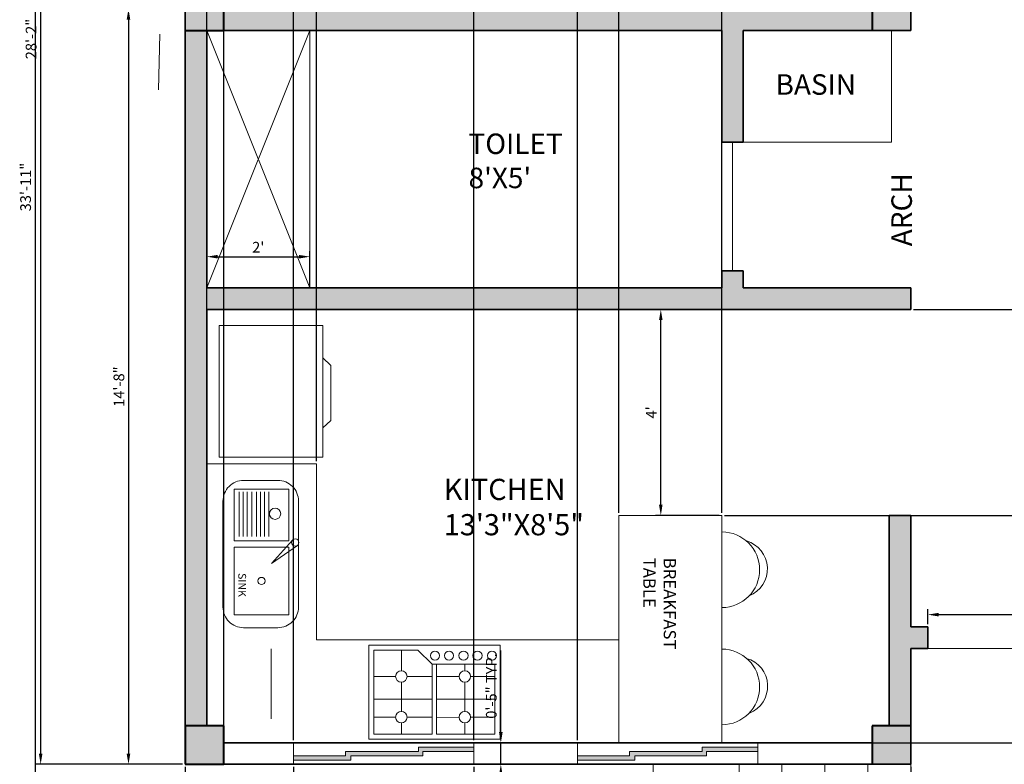
# Model space of a CAD drawing. Units: inches. Extents: x 918 to 1328, y 603 to 1174.
# Tile 2 of 4: x 918 to 1147, y 798 to 972. Entities that reach past the tile are written whole.
import ezdxf

# ---------------------------------------------------------------- set-up
doc = ezdxf.new("R2010")
doc.units = ezdxf.units.IN
for name, color, linetype, lineweight in [('A-ANNO-DIMS', 1, 'Continuous', 18), ('A-ANNO-TEXT', 7, 'Continuous', 18), ('A-COLS', 7, 'Continuous', 40), ('A-DETL', 8, 'Continuous', 13), ('A-DOOR', 4, 'Continuous', 18), ('A-FLOR-CASE', 8, 'Continuous', 20), ('A-FURN', 8, 'Continuous', 18), ('A-GLAZ', 4, 'Continuous', 18), ('A-GLAZ-PATT', 5, 'Continuous', 13), ('A-WALL', 7, 'Continuous', 35), ('A-WALL-PATT', 7, 'Continuous', 13)]:
    doc.layers.add(name, color=color, linetype=linetype, lineweight=lineweight)
for name, color, linetype, lineweight, true_color in [('A-AREA-IDEN', 251, 'Continuous', 20, 0x636466), ('A-COLS-PATT', 251, 'Continuous', 13, 0x636466), ('A-EQPM', 252, 'Continuous', 18, 0x939598), ('A-FLOR-FIXT', 252, 'Continuous', 18, 0x939598), ('A-FLOR-STRS', 251, 'Continuous', 20, 0x636466)]:
    doc.layers.add(name, color=color, linetype=linetype, lineweight=lineweight, true_color=true_color)
doc.styles.get("Standard").update_dxf_attribs({"font": 'arial.ttf'})
doc.dimstyles.new('ISO-25', dxfattribs={"dimtxt": 2.5, "dimasz": 2.5, "dimexe": 1.25, "dimexo": 0.625, "dimtad": 1, "dimdec": 0, "dimlunit": 3, "dimtxsty": 'Standard', "dimcen": 2.5, "dimadec": 0, "dimazin": 0, "dimtfac": 1, "dimtdec": 0, "dimtmove": 0, "dimatfit": 3, "dimfxl": 1, "dimarcsym": 0})

# ---------------------------------------------------------------- blocks, each defined once
blk = doc.blocks.new('*D2')
at = {"layer": 'A-ANNO-DIMS', "color": 0, "lineweight": -2, "transparency": 16777216}
for p, q in [((955.86, 1136.24), (921.53, 1136.24)), ((922.78, 1133.74), (922.78, 800.74)), ((955.86, 798.24), (921.53, 798.24))]:
    blk.add_line(p, q, dxfattribs=at)
at = {"layer": 'A-ANNO-DIMS', "color": 0, "transparency": 16777216}
for points in [[(922.37, 1133.74), (923.2, 1133.74), (922.78, 1136.24)], [(922.37, 800.74), (923.2, 800.74), (922.78, 798.24)]]:
    blk.add_solid(points, dxfattribs=at)
at = {"layer": 'Defpoints', "color": 0, "transparency": 16777216}
for p in [(956.48, 1136.24), (922.78, 798.24), (956.48, 798.24)]:
    blk.add_point(p, dxfattribs=at)
at = {"layer": 'A-ANNO-DIMS', "color": 0, "transparency": 16777216, "insert": (920.88, 967.24), "char_height": 2.5, "attachment_point": 5, "rotation": 90}
blk.add_mtext('28\'-2"', dxfattribs=at)
blk = doc.blocks.new('*D3')
at = {"layer": 'A-ANNO-DIMS', "color": 0, "lineweight": -2, "transparency": 16777216}
for p, q in [((961.48, 909.87), (961.48, 917.77)), ((985.48, 909.87), (985.48, 917.77)), ((963.98, 916.52), (982.98, 916.52))]:
    blk.add_line(p, q, dxfattribs=at)
at = {"layer": 'A-ANNO-DIMS', "color": 0, "transparency": 16777216}
for points in [[(963.98, 916.93), (963.98, 916.1), (961.48, 916.52)], [(982.98, 916.93), (982.98, 916.1), (985.48, 916.52)]]:
    blk.add_solid(points, dxfattribs=at)
at = {"layer": 'Defpoints', "color": 0, "transparency": 16777216}
for p in [(985.48, 916.52), (961.48, 909.24), (985.48, 909.24)]:
    blk.add_point(p, dxfattribs=at)
at = {"layer": 'A-ANNO-DIMS', "color": 0, "transparency": 16777216, "insert": (973.48, 918.4), "char_height": 2.5, "attachment_point": 5}
blk.add_mtext("2'", dxfattribs=at)
blk = doc.blocks.new('*D8')
at = {"layer": 'A-ANNO-DIMS', "color": 0, "lineweight": -2, "transparency": 16777216}
for p, q in [((955.86, 974.24), (941.99, 974.24)), ((943.24, 971.74), (943.24, 800.74)), ((955.86, 798.24), (941.99, 798.24))]:
    blk.add_line(p, q, dxfattribs=at)
at = {"layer": 'A-ANNO-DIMS', "color": 0, "transparency": 16777216}
for points in [[(942.82, 971.74), (943.66, 971.74), (943.24, 974.24)], [(942.82, 800.74), (943.66, 800.74), (943.24, 798.24)]]:
    blk.add_solid(points, dxfattribs=at)
at = {"layer": 'Defpoints', "color": 0, "transparency": 16777216}
for p in [(956.48, 974.24), (943.24, 798.24), (956.48, 798.24)]:
    blk.add_point(p, dxfattribs=at)
at = {"layer": 'A-ANNO-DIMS', "color": 0, "transparency": 16777216, "insert": (941.34, 886.24), "char_height": 2.5, "attachment_point": 5, "rotation": 90}
blk.add_mtext('14\'-8"', dxfattribs=at)
blk = doc.blocks.new('*D11')
at = {"layer": 'A-ANNO-DIMS', "color": 0, "lineweight": -2, "transparency": 16777216}
for p, q in [((956.48, 797.62), (956.48, 707.87)), ((1125.48, 797.62), (1125.48, 707.87)), ((958.98, 709.12), (1122.98, 709.12))]:
    blk.add_line(p, q, dxfattribs=at)
at = {"layer": 'A-ANNO-DIMS', "color": 0, "transparency": 16777216}
for points in [[(958.98, 709.53), (958.98, 708.7), (956.48, 709.12)], [(1122.98, 709.53), (1122.98, 708.7), (1125.48, 709.12)]]:
    blk.add_solid(points, dxfattribs=at)
at = {"layer": 'Defpoints', "color": 0, "transparency": 16777216}
for p in [(956.48, 798.24), (1125.48, 798.24), (1125.48, 709.12)]:
    blk.add_point(p, dxfattribs=at)
at = {"layer": 'A-ANNO-DIMS', "color": 0, "transparency": 16777216, "insert": (1040.98, 711), "char_height": 2.5, "attachment_point": 5}
blk.add_mtext('14\'-1"', dxfattribs=at)
blk = doc.blocks.new('*D17')
at = {"layer": 'A-ANNO-DIMS', "color": 0, "lineweight": -2, "transparency": 16777216}
for p, q in [((1129.48, 830.87), (1129.48, 834.37)), ((1131.98, 833.12), (1174.98, 833.12)), ((1177.48, 830.87), (1177.48, 834.37))]:
    blk.add_line(p, q, dxfattribs=at)
at = {"layer": 'A-ANNO-DIMS', "color": 0, "transparency": 16777216}
for points in [[(1131.98, 833.53), (1131.98, 832.7), (1129.48, 833.12)], [(1174.98, 833.53), (1174.98, 832.7), (1177.48, 833.12)]]:
    blk.add_solid(points, dxfattribs=at)
at = {"layer": 'Defpoints', "color": 0, "transparency": 16777216}
for p in [(1177.48, 833.12), (1129.48, 830.24), (1177.48, 830.24)]:
    blk.add_point(p, dxfattribs=at)
at = {"layer": 'A-ANNO-DIMS', "color": 0, "transparency": 16777216, "insert": (1153.48, 834.99), "char_height": 2.5, "attachment_point": 5}
blk.add_mtext("4'", dxfattribs=at)
blk = doc.blocks.new('*D18')
at = {"layer": 'A-ANNO-DIMS', "color": 0, "lineweight": -2, "transparency": 16777216}
for p, q in [((1080.86, 904.24), (1066.01, 904.24)), ((1067.26, 858.74), (1067.26, 901.74)), ((1080.86, 856.24), (1066.01, 856.24))]:
    blk.add_line(p, q, dxfattribs=at)
at = {"layer": 'A-ANNO-DIMS', "color": 0, "transparency": 16777216}
for points in [[(1066.84, 901.74), (1067.67, 901.74), (1067.26, 904.24)], [(1066.84, 858.74), (1067.67, 858.74), (1067.26, 856.24)]]:
    blk.add_solid(points, dxfattribs=at)
at = {"layer": 'Defpoints', "color": 0, "transparency": 16777216}
for p in [(1067.26, 904.24), (1081.48, 904.24), (1081.48, 856.24)]:
    blk.add_point(p, dxfattribs=at)
at = {"layer": 'A-ANNO-DIMS', "color": 0, "transparency": 16777216, "insert": (1065.38, 880.24), "char_height": 2.5, "attachment_point": 5, "rotation": 90}
blk.add_mtext("4'", dxfattribs=at)
blk = doc.blocks.new('WIN-SLIDING-42')
for p, q in [((0, 5), (0, 0)), ((42, 5), (0, 5)), ((42, 0), (42, 5)), ((12.14, 3), (29.09, 3)), ((12.14, 1.97), (12.14, 3)), ((29.09, 3), (29.09, 4.02)), ((29.09, 4.02), (42, 4.02)), ((30.11, 1.97), (30.11, 3)), ((30.11, 3), (42, 3)), ((0, 1.97), (12.14, 1.97)), ((0, 0.97), (13.35, 0.97)), ((0, 0), (42, 0)), ((13.35, 0.97), (13.35, 1.97)), ((13.35, 1.97), (30.11, 1.97))]:
    blk.add_line(p, q)
blk = doc.blocks.new('*D32')
at = {"layer": 'A-ANNO-DIMS', "color": 0, "lineweight": -2, "transparency": 16777216}
for p, q in [((981.69, 797.62), (981.69, 790.69)), ((1023.69, 797.62), (1023.69, 790.69)), ((984.19, 791.94), (1021.19, 791.94)), ((1023.69, 791.94), (1073.9, 791.94))]:
    blk.add_line(p, q, dxfattribs=at)
at = {"layer": 'A-ANNO-DIMS', "color": 0, "transparency": 16777216}
for points in [[(984.19, 792.36), (984.19, 791.53), (981.69, 791.94)], [(1021.19, 792.36), (1021.19, 791.53), (1023.69, 791.94)]]:
    blk.add_solid(points, dxfattribs=at)
at = {"layer": 'Defpoints', "color": 0, "transparency": 16777216}
for p in [(981.69, 798.24), (1023.69, 798.24), (1023.69, 791.94)]:
    blk.add_point(p, dxfattribs=at)
at = {"layer": 'A-ANNO-DIMS', "color": 0, "transparency": 16777216, "insert": (1050.05, 793.86), "char_height": 2.5, "attachment_point": 5}
blk.add_mtext('SLIDING WINDOW 3\'-6" TYP.', dxfattribs=at)
blk = doc.blocks.new('*D33')
at = {"layer": 'A-ANNO-DIMS', "color": 0, "lineweight": -2, "transparency": 16777216}
for p, q in [((1029.99, 805.74), (1029.99, 824.73)), ((1024.31, 803.24), (1031.24, 803.24)), ((1029.99, 798.24), (1029.99, 803.24)), ((1024.31, 798.24), (1031.24, 798.24)), ((1029.99, 795.74), (1029.99, 793.24))]:
    blk.add_line(p, q, dxfattribs=at)
at = {"layer": 'A-ANNO-DIMS', "color": 0, "transparency": 16777216}
for points in [[(1029.57, 805.74), (1030.41, 805.74), (1029.99, 803.24)], [(1029.57, 795.74), (1030.41, 795.74), (1029.99, 798.24)]]:
    blk.add_solid(points, dxfattribs=at)
at = {"layer": 'Defpoints', "color": 0, "transparency": 16777216}
for p in [(1023.69, 803.24), (1029.99, 803.24), (1023.69, 798.24)]:
    blk.add_point(p, dxfattribs=at)
at = {"layer": 'A-ANNO-DIMS', "color": 0, "transparency": 16777216, "insert": (1028.09, 816.49), "char_height": 2.5, "attachment_point": 5, "rotation": 90}
blk.add_mtext('0\'-5" TYP.', dxfattribs=at)
blk = doc.blocks.new('*D44')
at = {"layer": 'A-ANNO-DIMS', "color": 0, "lineweight": -2, "transparency": 16777216}
for p, q in [((955.86, 1136.24), (920.25, 1136.24)), ((921.5, 1133.74), (921.5, 731.74)), ((1064.86, 729.24), (920.25, 729.24))]:
    blk.add_line(p, q, dxfattribs=at)
at = {"layer": 'A-ANNO-DIMS', "color": 0, "transparency": 16777216}
for points in [[(921.09, 1133.74), (921.92, 1133.74), (921.5, 1136.24)], [(921.09, 731.74), (921.92, 731.74), (921.5, 729.24)]]:
    blk.add_solid(points, dxfattribs=at)
at = {"layer": 'Defpoints', "color": 0, "transparency": 16777216}
for p in [(956.48, 1136.24), (921.5, 729.24), (1065.48, 729.24)]:
    blk.add_point(p, dxfattribs=at)
at = {"layer": 'A-ANNO-DIMS', "color": 0, "transparency": 16777216, "insert": (919.6, 932.74), "char_height": 2.5, "attachment_point": 5, "rotation": 90}
blk.add_mtext('33\'-11"', dxfattribs=at)
blk = doc.blocks.new('*D47')
at = {"layer": 'A-ANNO-DIMS', "color": 0, "lineweight": -2, "transparency": 16777216}
for p, q in [((965.48, 803.87), (965.48, 1166.19)), ((981.69, 803.87), (981.69, 1166.19)), ((967.98, 1164.94), (979.19, 1164.94))]:
    blk.add_line(p, q, dxfattribs=at)
at = {"layer": 'A-ANNO-DIMS', "color": 0, "transparency": 16777216}
for points in [[(967.98, 1165.36), (967.98, 1164.53), (965.48, 1164.94)], [(979.19, 1165.36), (979.19, 1164.53), (981.69, 1164.94)]]:
    blk.add_solid(points, dxfattribs=at)
at = {"layer": 'Defpoints', "color": 0, "transparency": 16777216}
for p in [(981.69, 1164.94), (965.48, 803.24), (981.69, 803.24)]:
    blk.add_point(p, dxfattribs=at)
at = {"layer": 'A-ANNO-DIMS', "color": 0, "transparency": 16777216, "insert": (973.59, 1166.82), "char_height": 2.5, "attachment_point": 5}
blk.add_mtext('1\'-4"', dxfattribs=at)
blk = doc.blocks.new('*D48')
at = {"layer": 'A-ANNO-DIMS', "color": 0, "lineweight": -2, "transparency": 16777216}
for p, q in [((1023.69, 803.87), (1023.69, 1166.19)), ((1047.83, 803.87), (1047.83, 1166.19)), ((1026.19, 1164.94), (1045.33, 1164.94))]:
    blk.add_line(p, q, dxfattribs=at)
at = {"layer": 'A-ANNO-DIMS', "color": 0, "transparency": 16777216}
for points in [[(1026.19, 1165.36), (1026.19, 1164.53), (1023.69, 1164.94)], [(1045.33, 1165.36), (1045.33, 1164.53), (1047.83, 1164.94)]]:
    blk.add_solid(points, dxfattribs=at)
at = {"layer": 'Defpoints', "color": 0, "transparency": 16777216}
for p in [(1047.83, 1164.94), (1023.69, 803.24), (1047.83, 803.24)]:
    blk.add_point(p, dxfattribs=at)
at = {"layer": 'A-ANNO-DIMS', "color": 0, "transparency": 16777216, "insert": (1035.76, 1166.84), "char_height": 2.5, "attachment_point": 5}
blk.add_mtext('2\'-0"', dxfattribs=at)
blk = doc.blocks.new('*D51')
at = {"layer": 'A-ANNO-DIMS', "color": 0, "lineweight": -2, "transparency": 16777216}
for p, q in [((1126.11, 904.24), (1321.43, 904.24)), ((1320.18, 901.74), (1320.18, 858.74)), ((1126.11, 856.24), (1321.43, 856.24))]:
    blk.add_line(p, q, dxfattribs=at)
at = {"layer": 'A-ANNO-DIMS', "color": 0, "transparency": 16777216}
for points in [[(1319.77, 901.74), (1320.6, 901.74), (1320.18, 904.24)], [(1319.77, 858.74), (1320.6, 858.74), (1320.18, 856.24)]]:
    blk.add_solid(points, dxfattribs=at)
at = {"layer": 'Defpoints', "color": 0, "transparency": 16777216}
for p in [(1125.48, 904.24), (1125.48, 856.24), (1320.18, 856.24)]:
    blk.add_point(p, dxfattribs=at)
at = {"layer": 'A-ANNO-DIMS', "color": 0, "transparency": 16777216, "insert": (1318.28, 880.24), "char_height": 2.5, "attachment_point": 5, "rotation": 90}
blk.add_mtext('4\'-0"', dxfattribs=at)
blk = doc.blocks.new('*D54')
at = {"layer": 'A-ANNO-DIMS', "color": 0, "lineweight": -2, "transparency": 16777216}
for p, q in [((961.48, 868.87), (961.48, 1166.19)), ((987.08, 868.87), (987.08, 1166.19)), ((963.98, 1164.94), (984.58, 1164.94))]:
    blk.add_line(p, q, dxfattribs=at)
at = {"layer": 'A-ANNO-DIMS', "color": 0, "transparency": 16777216}
for points in [[(963.98, 1165.36), (963.98, 1164.53), (961.48, 1164.94)], [(984.58, 1165.36), (984.58, 1164.53), (987.08, 1164.94)]]:
    blk.add_solid(points, dxfattribs=at)
at = {"layer": 'Defpoints', "color": 0, "transparency": 16777216}
for p in [(987.08, 1164.94), (961.48, 868.24), (987.08, 868.24)]:
    blk.add_point(p, dxfattribs=at)
at = {"layer": 'A-ANNO-DIMS', "color": 0, "transparency": 16777216, "insert": (974.28, 1166.86), "char_height": 2.5, "attachment_point": 5}
blk.add_mtext('2\'-1 1/2"', dxfattribs=at)
blk = doc.blocks.new('*D55')
at = {"layer": 'A-ANNO-DIMS', "color": 0, "lineweight": -2, "transparency": 16777216}
for p, q in [((1057.48, 856.87), (1057.48, 1166.19)), ((1081.48, 856.87), (1081.48, 1166.19)), ((1059.98, 1164.94), (1078.98, 1164.94))]:
    blk.add_line(p, q, dxfattribs=at)
at = {"layer": 'A-ANNO-DIMS', "color": 0, "transparency": 16777216}
for points in [[(1059.98, 1165.36), (1059.98, 1164.53), (1057.48, 1164.94)], [(1078.98, 1165.36), (1078.98, 1164.53), (1081.48, 1164.94)]]:
    blk.add_solid(points, dxfattribs=at)
at = {"layer": 'Defpoints', "color": 0, "transparency": 16777216}
for p in [(1081.48, 1164.94), (1057.48, 856.24), (1081.48, 856.24)]:
    blk.add_point(p, dxfattribs=at)
at = {"layer": 'A-ANNO-DIMS', "color": 0, "transparency": 16777216, "insert": (1069.48, 1166.84), "char_height": 2.5, "attachment_point": 5}
blk.add_mtext('2\'-0"', dxfattribs=at)
blk = doc.blocks.new('*D56')
at = {"layer": 'A-ANNO-DIMS', "color": 0, "lineweight": -2, "transparency": 16777216}
for p, q in [((1082.11, 856.24), (1321.43, 856.24)), ((1320.18, 853.74), (1320.18, 805.74)), ((1082.11, 803.24), (1321.43, 803.24))]:
    blk.add_line(p, q, dxfattribs=at)
at = {"layer": 'A-ANNO-DIMS', "color": 0, "transparency": 16777216}
for points in [[(1319.77, 853.74), (1320.6, 853.74), (1320.18, 856.24)], [(1319.77, 805.74), (1320.6, 805.74), (1320.18, 803.24)]]:
    blk.add_solid(points, dxfattribs=at)
at = {"layer": 'Defpoints', "color": 0, "transparency": 16777216}
for p in [(1081.48, 856.24), (1081.48, 803.24), (1320.18, 803.24)]:
    blk.add_point(p, dxfattribs=at)
at = {"layer": 'A-ANNO-DIMS', "color": 0, "transparency": 16777216, "insert": (1318.29, 829.74), "char_height": 2.5, "attachment_point": 5, "rotation": 90}
blk.add_mtext('4\'-5"', dxfattribs=at)

msp = doc.modelspace()

# ---------------------------------------------------------------- hatches: boundary and pattern name
at = {"layer": 'A-COLS-PATT'}
h = msp.add_hatch(color=256, dxfattribs=at)
h.dxf.hatch_style = 1
h.paths.add_polyline_path([(965.48, 1136.24), (956.48, 1136.24), (956.48, 1127.24), (965.48, 1127.24)])
h.paths.add_polyline_path([(1125.48, 1136.24), (1116.48, 1136.24), (1116.48, 1127.24), (1125.48, 1127.24)])
h.paths.add_polyline_path([(1291.48, 1136.24), (1282.48, 1136.24), (1282.48, 1127.24), (1291.48, 1127.24)])
h.paths.add_polyline_path([(1125.48, 978.24), (1116.48, 978.24), (1116.48, 969.24), (1125.48, 969.24)])
h.paths.add_polyline_path([(965.48, 978.24), (956.48, 978.24), (956.48, 969.24), (965.48, 969.24)])
h.paths.add_polyline_path([(965.48, 807.24), (956.48, 807.24), (956.48, 798.24), (965.48, 798.24)])
h.paths.add_polyline_path([(1125.48, 807.24), (1116.48, 807.24), (1116.48, 798.24), (1125.48, 798.24)])
h.paths.add_polyline_path([(1291.48, 807.24), (1282.48, 807.24), (1282.48, 798.24), (1291.48, 798.24)])
h.paths.add_polyline_path([(1291.48, 1030.24), (1282.48, 1030.24), (1282.48, 1021.24), (1291.48, 1021.24)])
h.paths.add_polyline_path([(1291.48, 978.24), (1282.48, 978.24), (1282.48, 969.24), (1291.48, 969.24)])
at = {"layer": 'A-GLAZ-PATT'}
h = msp.add_hatch(color=256, dxfattribs=at)
h.dxf.hatch_style = 1
h.paths.add_polyline_path([(995.04, 800.21), (1011.8, 800.21), (1011.8, 801.25), (1023.69, 801.25), (1023.69, 802.26), (1010.78, 802.26), (1010.78, 801.25), (993.83, 801.25), (993.83, 800.21), (981.69, 800.21), (981.69, 799.22), (995.04, 799.22)])
h.paths.add_polyline_path([(1061.18, 800.21), (1077.94, 800.21), (1077.94, 801.25), (1089.83, 801.25), (1089.83, 802.26), (1076.92, 802.26), (1076.92, 801.25), (1059.97, 801.25), (1059.97, 800.21), (1047.83, 800.21), (1047.83, 799.22), (1061.18, 799.22)])
at = {"layer": 'A-WALL-PATT'}
h = msp.add_hatch(color=256, dxfattribs=at)
h.dxf.hatch_style = 1
h.paths.add_polyline_path([(961.48, 969.24), (956.48, 969.24), (956.48, 807.24), (961.48, 807.24), (961.48, 904.24), (1125.48, 904.24), (1125.48, 909.24), (1086.48, 909.24), (1086.48, 913.24), (1081.48, 913.24), (1081.48, 909.24), (961.48, 909.24)])
h.paths.add_polyline_path([(1116.48, 974.24), (965.48, 974.24), (965.48, 969.24), (1081.48, 969.24), (1081.48, 943.24), (1086.48, 943.24), (1086.48, 969.24), (1116.48, 969.24)])
h.paths.add_polyline_path([(1004.98, 1136.24), (965.48, 1136.24), (965.48, 1131.24), (1004.98, 1131.24)])
h.paths.add_polyline_path([(1116.48, 1136.24), (1076.98, 1136.24), (1076.98, 1131.24), (1116.48, 1131.24)])
h.paths.add_polyline_path([(1176.26, 1136.24), (1125.48, 1136.24), (1125.48, 1131.24), (1176.26, 1131.24)])
h.paths.add_polyline_path([(1282.48, 1136.24), (1248.26, 1136.24), (1248.26, 1131.24), (1282.48, 1131.24)])
h.paths.add_polyline_path([(1125.48, 1127.24), (1120.48, 1127.24), (1120.48, 1025.24), (1125.48, 1025.24)])
h.paths.add_polyline_path([(1291.48, 1035.24), (1168.48, 1035.24), (1168.48, 1030.24), (1291.48, 1030.24)])
h.paths.add_polyline_path([(1125.48, 825.24), (1129.48, 825.24), (1129.48, 830.24), (1125.48, 830.24), (1125.48, 856.24), (1120.48, 856.24), (1120.48, 807.24), (1125.48, 807.24)])
h.paths.add_polyline_path([(1191.92, 830.24), (1177.48, 830.24), (1177.48, 825.24), (1191.92, 825.24)])
h.paths.add_polyline_path([(1291.48, 969.24), (1286.48, 969.24), (1286.48, 830.24), (1263.92, 830.24), (1263.92, 825.24), (1286.48, 825.24), (1286.48, 807.24), (1291.48, 807.24)])
h.paths.add_polyline_path([(1291.48, 1021.24), (1286.48, 1021.24), (1286.48, 978.24), (1291.48, 978.24)])
h.paths.add_polyline_path([(1291.48, 1127.24), (1286.48, 1127.24), (1286.48, 1035.24), (1291.48, 1035.24)])

# ---------------------------------------------------------------- linework, layer by layer
at = {"layer": 'A-COLS'}
for p, q in [((965.48, 969.24), (965.48, 978.24)), ((1116.48, 978.24), (1116.48, 969.24)), ((956.48, 969.24), (965.48, 969.24)), ((965.48, 807.24), (956.48, 807.24)), ((956.48, 807.24), (956.48, 798.24)), ((965.48, 798.24), (965.48, 807.24)), ((1125.48, 807.24), (1116.48, 807.24)), ((1116.48, 807.24), (1116.48, 798.24)), ((956.48, 798.24), (965.48, 798.24))]:
    msp.add_line(p, q, dxfattribs=at)
at = {"layer": 'A-DETL'}
for p, q in [((950.2, 955.4), (950.51, 968.39)), ((976.49, 808.83), (976.49, 825.14))]:
    msp.add_line(p, q, dxfattribs=at)
at = {"layer": 'A-DOOR'}
for p, q in [((1083.98, 943.24), (1083.98, 913.24)), ((1129.48, 825.24), (1177.48, 825.24))]:
    msp.add_line(p, q, dxfattribs=at)
at = {"layer": 'A-EQPM'}
for p, q in [((988.51, 892.92), (990.42, 891.15)), ((990.42, 891.15), (990.42, 878.39)), ((990.42, 878.39), (988.51, 876.62)), ((1010.63, 824.81), (1000.39, 824.81)), ((1000.39, 824.81), (1000.39, 805.25)), ((1006.81, 820.05), (1006.81, 824.81)), ((1014.01, 821.6), (1010.63, 824.81)), ((1014.01, 805.25), (1014.01, 821.6)), ((1014.01, 821.6), (1028.62, 821.6)), ((1015.02, 805.25), (1015.02, 821.6)), ((1021.6, 820.05), (1021.6, 821.6)), ((1028.62, 805.25), (1028.62, 821.6)), ((1005.49, 818.72), (1000.39, 818.72)), ((1006.81, 817.4), (1006.81, 810.57)), ((1008.14, 818.72), (1014.01, 818.72)), ((1015.02, 818.72), (1020.28, 818.72)), ((1021.6, 817.4), (1021.6, 810.57)), ((1022.93, 818.72), (1028.62, 818.72)), ((1000.39, 813.42), (1014.01, 813.42)), ((1015.02, 813.42), (1028.62, 813.42)), ((1005.49, 809.24), (1000.39, 809.24)), ((1006.81, 807.92), (1006.81, 805.25)), ((1008.14, 809.24), (1014.01, 809.21)), ((1015.02, 809.21), (1020.31, 809.18)), ((1021.6, 807.92), (1021.6, 805.25)), ((1022.93, 809.24), (1028.62, 809.24)), ((1000.39, 805.25), (1014.01, 805.25)), ((1015.02, 805.25), (1028.62, 805.25))]:
    msp.add_line(p, q, dxfattribs=at)
for points in [[(964.39, 869.83), (988.51, 869.83), (988.51, 900.48), (964.39, 900.48)], [(999.21, 804.07), (1029.8, 804.07), (1029.8, 825.99), (999.21, 825.99)]]:
    msp.add_lwpolyline(points, close=True, dxfattribs=at)
for centre, radius in [((1014.64, 823.57), 1.07), ((1017.93, 823.57), 1.07), ((1021.29, 823.57), 1.07), ((1024.56, 823.57), 1.07), ((1027.93, 823.57), 1.07), ((1006.81, 818.72), 1.33), ((1021.6, 818.72), 1.33), ((1006.81, 809.24), 1.33), ((1021.6, 809.24), 1.33)]:
    msp.add_circle(centre, radius, dxfattribs=at)
at = {"layer": 'A-FLOR-CASE'}
for p, q in [((987.08, 868.24), (961.48, 868.24)), ((987.08, 868.24), (987.08, 827.24)), ((987.08, 827.24), (1057.48, 827.24)), ((1057.48, 827.24), (1057.48, 803.24))]:
    msp.add_line(p, q, dxfattribs=at)
at = {"layer": 'A-FLOR-FIXT'}
for p, q in [((961.48, 909.24), (985.48, 969.24)), ((961.48, 969.24), (985.48, 909.24)), ((985.48, 969.24), (985.48, 909.24)), ((1120.98, 943.24), (1120.98, 969.24)), ((1086.48, 943.24), (1120.98, 943.24)), ((967.86, 850.3), (967.86, 862.34)), ((967.86, 862.34), (980.6, 862.34)), ((969.01, 851.35), (969.01, 861.72)), ((969.97, 851.35), (969.97, 861.72)), ((970.92, 851.35), (970.92, 861.72)), ((971.97, 851.35), (971.97, 861.72)), ((973.06, 851.35), (973.06, 861.72)), ((974.02, 851.35), (974.02, 861.72)), ((974.93, 851.35), (974.93, 861.72)), ((975.97, 851.35), (975.97, 861.72)), ((980.6, 862.34), (980.6, 850.3)), ((980.6, 850.3), (967.86, 850.3)), ((976.58, 845), (981.47, 850.47)), ((976.58, 845), (982.59, 849.22)), ((970.06, 830.07), (978.04, 830.07))]:
    msp.add_line(p, q, dxfattribs=at)
for points in [[(970.06, 864.4), (978.21, 864.4)], [(965.25, 834.88), (965.25, 859.58)], [(982.85, 859.59), (982.85, 834.88)]]:
    msp.add_lwpolyline(points, dxfattribs=at)
msp.add_lwpolyline([(980.6, 833.07), (967.86, 833.07), (967.86, 848.85), (980.6, 848.85)], close=True, dxfattribs=at)
for centre, radius in [((977.38, 856.63), 1.32), ((982.1, 849.91), 0.846), ((974.23, 840.96), 0.846)]:
    msp.add_circle(centre, radius, dxfattribs=at)
for centre, start, end in [((970.06, 859.58), 89.9635, 180), ((978.04, 859.59), 359.9635, 90), ((970.06, 834.88), 180, 270.0365), ((978.04, 834.88), 270, 0.0365)]:
    msp.add_arc(centre, 4.81, start, end, dxfattribs=at)
at = {"layer": 'A-FLOR-STRS'}
for p, q in [((1065.48, 798.24), (1065.48, 729.24)), ((1085.48, 798.24), (1085.48, 729.24)), ((1095.48, 798.24), (1095.48, 729.24)), ((1105.48, 798.24), (1105.48, 729.24)), ((1115.48, 798.24), (1115.48, 729.24)), ((1125.48, 798.24), (1125.48, 729.24))]:
    msp.add_line(p, q, dxfattribs=at)
at = {"layer": 'A-FURN'}
for p, q in [((1081.48, 856.24), (1057.48, 856.24)), ((1057.48, 856.24), (1057.48, 827.24)), ((1081.48, 803.24), (1081.48, 856.24)), ((1057.48, 803.24), (1081.48, 803.24))]:
    msp.add_line(p, q, dxfattribs=at)
for centre, radius, start, end in [((1081.48, 843.58), 8.81, 270, 90), ((1085.33, 843.77), 6.77, 291.7552, 74.0331), ((1081.48, 816.27), 8.81, 270, 90), ((1085.38, 816.42), 6.77, 291.7552, 74.0331)]:
    msp.add_arc(centre, radius, start, end, dxfattribs=at)
at = {"layer": 'A-WALL'}
for p, q in [((956.48, 1136.24), (956.48, 798.24)), ((1125.48, 983.79), (1125.48, 969.24)), ((1081.48, 969.24), (956.48, 969.24)), ((961.48, 969.24), (961.48, 909.24)), ((1081.48, 969.24), (1081.48, 943.24)), ((1086.48, 969.24), (1086.48, 943.24)), ((1125.48, 969.24), (1086.48, 969.24)), ((1086.48, 943.24), (1081.48, 943.24)), ((1086.48, 913.24), (1081.48, 913.24)), ((1081.48, 913.24), (1081.48, 909.24)), ((1086.48, 913.24), (1086.48, 909.24)), ((1081.48, 909.24), (961.48, 909.24)), ((1125.48, 909.24), (1086.48, 909.24)), ((1125.48, 909.24), (1125.48, 904.24)), ((961.48, 904.24), (961.48, 807.24)), ((1125.48, 904.24), (961.48, 904.24)), ((1120.48, 856.24), (1120.48, 807.24)), ((1120.48, 856.24), (1125.48, 856.24)), ((1125.48, 856.24), (1125.48, 830.24)), ((1129.48, 830.24), (1125.48, 830.24)), ((1129.48, 825.24), (1129.48, 830.24)), ((1125.48, 825.24), (1125.48, 798.24)), ((1129.48, 825.24), (1125.48, 825.24)), ((965.48, 803.24), (1116.48, 803.24)), ((956.48, 798.24), (1125.48, 798.24))]:
    msp.add_line(p, q, dxfattribs=at)

# ---------------------------------------------------------------- block references
at = {"layer": 'A-GLAZ'}
for p in [(981.69, 798.24), (1047.83, 798.24)]:
    msp.add_blockref('WIN-SLIDING-42', p, dxfattribs=at)

# ---------------------------------------------------------------- texts
at = {"layer": 'A-ANNO-TEXT', "attachment_point": 1}
for s, width, gutter_width, insert, char_height, rotation in [('ARCH', 21.0887, 14.8, (1120.98, 918.95), 4.778, 90), ('BREAKFAST TABLE', 24.7502, 5.79, (1070.79, 846.38), 2.8543, 270), ('SINK', 4.5558, 9.04, (970.64, 842.81), 1.809, 270)]:
    msp.add_mtext_dynamic_manual_height_columns(s, width=width, gutter_width=gutter_width, heights=[0], dxfattribs=dict(at, insert=insert, char_height=char_height, rotation=rotation))
at = {"layer": 'A-AREA-IDEN', "attachment_point": 1}
for s, width, gutter_width, insert, char_height in [('BASIN', 26.7747, 24.41, (1093.99, 959.03), 4.778), ("TOILET\\P8'X5'", 64.8021, 26.2, (1022.47, 945.22), 4.778), ('KITCHEN\\P13\'3"X8\'5"', 72.5125, 24.67, (1016.7, 864.76), 4.933)]:
    msp.add_mtext_dynamic_manual_height_columns(s, width=width, gutter_width=gutter_width, heights=[0], dxfattribs=dict(at, insert=insert, char_height=char_height))

# ---------------------------------------------------------------- dimensions: what is measured, and where the dimension line sits
at = {"layer": 'A-ANNO-DIMS'}
for base, p1, p2, override, picture, middle in [((987.08, 1164.94), (961.48, 868.24), (987.08, 868.24), {"dimdec": 1, "dimlfac": 1, "dimrnd": 0, "dimzin": 1, "dimdsep": 46, "dimlunit": 4, "dimfrac": 2}, '*D54', (974.28, 1166.86)), ((981.69, 1164.94), (965.48, 803.24), (981.69, 803.24), {"dimdec": 1, "dimlfac": 1, "dimrnd": 0, "dimzin": 1, "dimdsep": 46, "dimlunit": 4, "dimfrac": 2}, '*D47', (973.59, 1166.82)), ((1047.83, 1164.94), (1023.69, 803.24), (1047.83, 803.24), {"dimdec": 1, "dimlfac": 1, "dimrnd": 0, "dimzin": 1, "dimdsep": 46, "dimlunit": 4, "dimfrac": 2}, '*D48', (1035.76, 1166.84)), ((1081.48, 1164.94), (1057.48, 856.24), (1081.48, 856.24), {"dimdec": 1, "dimlfac": 1, "dimrnd": 0, "dimzin": 1, "dimdsep": 46, "dimlunit": 4, "dimfrac": 2}, '*D55', (1069.48, 1166.84)), ((985.48, 916.52), (961.48, 909.24), (985.48, 909.24), {"dimclrd": 0, "dimclre": 0, "dimclrt": 0}, '*D3', (973.48, 918.4)), ((1177.48, 833.12), (1129.48, 830.24), (1177.48, 830.24), {"dimclrd": 0, "dimclre": 0, "dimclrt": 0}, '*D17', (1153.48, 834.99)), ((1125.48, 709.12), (956.48, 798.24), (1125.48, 798.24), {"dimclrd": 0, "dimclre": 0, "dimclrt": 0}, '*D11', (1040.98, 711))]:
    dim = msp.add_linear_dim(base=base, p1=p1, p2=p2, dimstyle='ISO-25', override=override, dxfattribs=at)
    dim.commit()
    dim.dimension.update_dxf_attribs({"geometry": picture, "text_midpoint": middle})
for base, p1, p2, override, picture, middle in [((921.5, 729.24), (956.48, 1136.24), (1065.48, 729.24), {"dimdec": 1, "dimlfac": 1, "dimrnd": 0, "dimzin": 1, "dimdsep": 46, "dimlunit": 4, "dimfrac": 2}, '*D44', (919.6, 932.74)), ((922.78, 798.24), (956.48, 1136.24), (956.48, 798.24), {"dimclrd": 0, "dimclre": 0, "dimclrt": 0}, '*D2', (920.88, 967.24)), ((943.24, 798.24), (956.48, 974.24), (956.48, 798.24), {"dimclrd": 0, "dimclre": 0, "dimclrt": 0}, '*D8', (941.34, 886.24)), ((1067.26, 904.24), (1081.48, 856.24), (1081.48, 904.24), {"dimclrd": 0, "dimclre": 0, "dimclrt": 0}, '*D18', (1065.38, 880.24)), ((1320.18, 856.24), (1125.48, 904.24), (1125.48, 856.24), {"dimdec": 1, "dimlfac": 1, "dimrnd": 0, "dimzin": 1, "dimdsep": 46, "dimlunit": 4, "dimfrac": 2}, '*D51', (1318.28, 880.24)), ((1320.18, 803.24), (1081.48, 856.24), (1081.48, 803.24), {"dimdec": 1, "dimlfac": 1, "dimrnd": 0, "dimzin": 1, "dimdsep": 46, "dimlunit": 4, "dimfrac": 2}, '*D56', (1318.29, 829.74))]:
    dim = msp.add_linear_dim(base=base, p1=p1, p2=p2, angle=90, dimstyle='ISO-25', override=override, dxfattribs=at)
    dim.commit()
    dim.dimension.update_dxf_attribs({"geometry": picture, "text_midpoint": middle})
dim = msp.add_linear_dim(base=(1029.99, 803.24), p1=(1023.69, 798.24), p2=(1023.69, 803.24), angle=90, text='<> TYP.', dimstyle='ISO-25', override={"dimdec": 1, "dimlfac": 1, "dimrnd": 0, "dimzin": 1, "dimdsep": 46, "dimlunit": 4, "dimfrac": 2}, dxfattribs=at)
dim.commit()
dim.dimension.update_dxf_attribs({"geometry": '*D33', "text_midpoint": (1028.09, 816.49)})
dim = msp.add_linear_dim(base=(1023.69, 791.94), p1=(981.69, 798.24), p2=(1023.69, 798.24), text='SLIDING WINDOW <> TYP.', dimstyle='ISO-25', override={"dimdec": 1, "dimlfac": 1, "dimrnd": 0, "dimzin": 1, "dimdsep": 46, "dimlunit": 4, "dimfrac": 2}, dxfattribs=at)
dim.commit()
dim.dimension.update_dxf_attribs({"geometry": '*D32', "text_midpoint": (1050.05, 793.86)})

doc.saveas('drawing.dxf')
